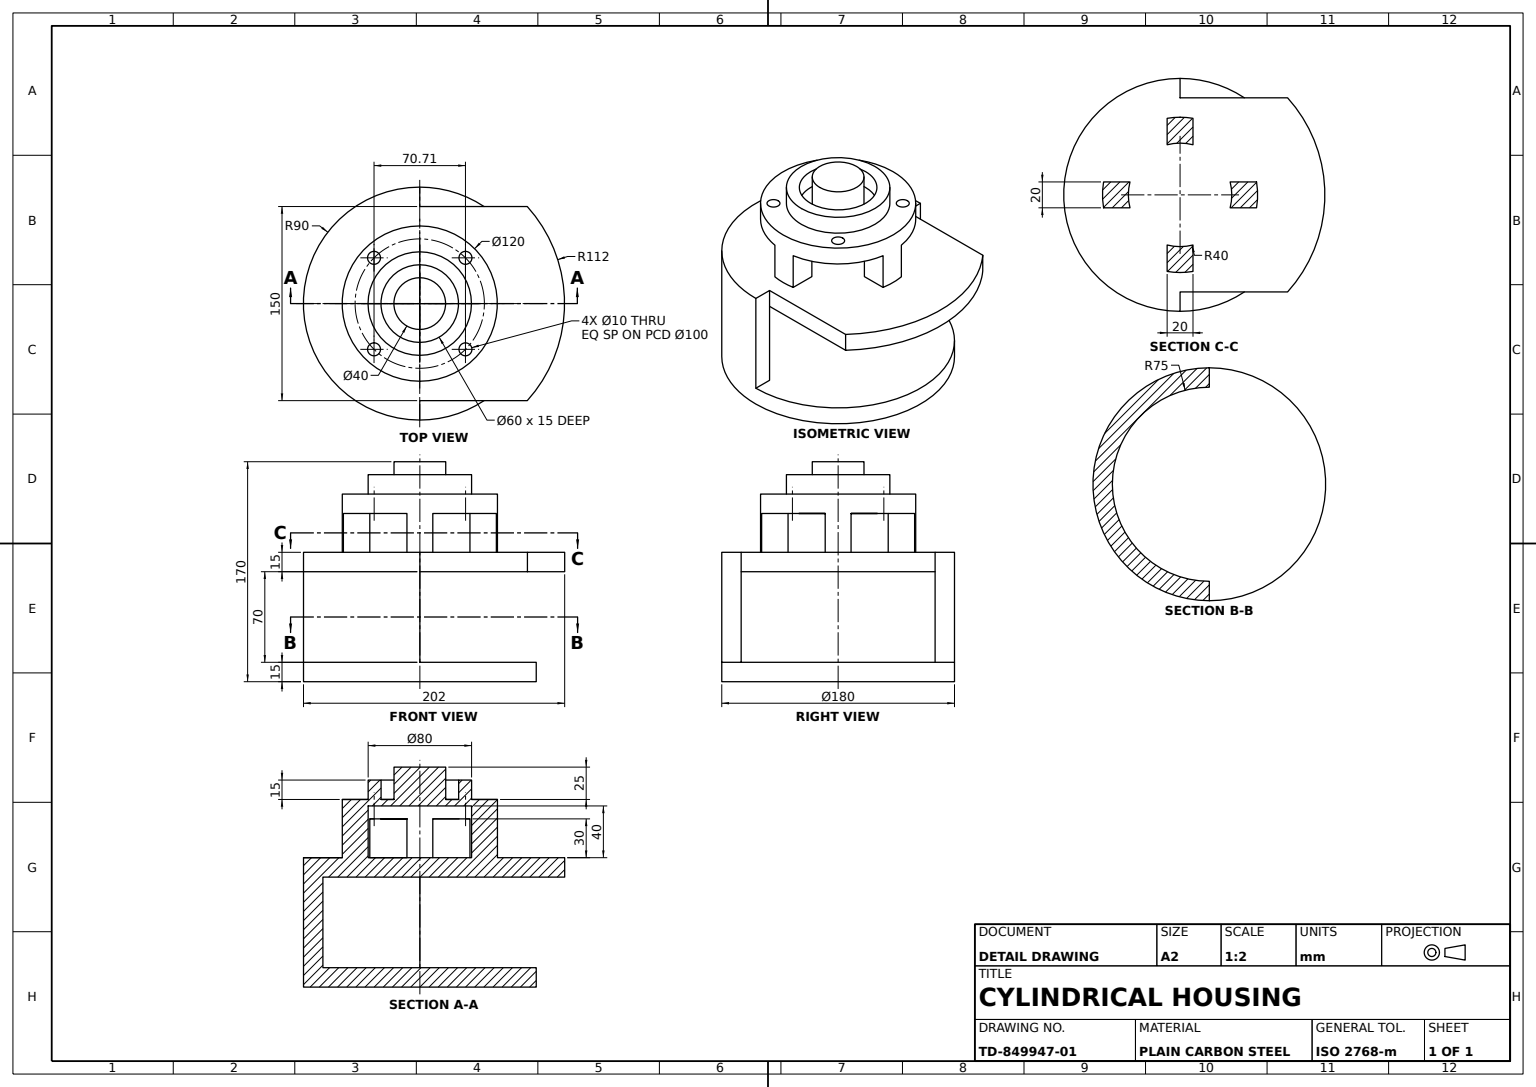
SolidWorks part; units mm, degrees
material "Plain Carbon Steel"
ref_plane "Front Plane" through (0, 0, 0) normal (0, 0, 1) x (1, 0, 0)
ref_plane "Top Plane" through (0, 0, 0) normal (0, 1, 0) x (1, 0, 0)
ref_plane "Right Plane" through (0, 0, 0) normal (1, 0, 0) x (0, 0, -1)
sketch "Base Disc Sketch" plane through (0, 0, 0) normal (0, 1, 0) x (1, 0, 0)
  circle A0 centre (0, 0) radius 90
  dimension "D1" = 180
extrude "Base Disc Ø180" add sketch "Base Disc Sketch" along normal blind 15
sketch "Clamp Frame Wall Sketch" plane through (0, 15, 0) normal (0, 1, 0) x (1, 0, 0)
  line L0 (0, -90) -> (0, -75)
  line L1 (0, 75) -> (0, 90)
  arc A0 (0, 90) -> (0, -90) centre (0, 0) ccw
  arc A1 (0, 75) -> (0, -75) centre (0, 0) ccw
  dimension "D1" = 150
  dimension "D2" = 180
extrude "Clamp Frame Wall" add sketch "Clamp Frame Wall Sketch" along normal blind 70
sketch "Top Jaw Sketch" plane through (0, 85, 0) normal (0, 1, 0) x (1, 0, 0)
  line L1 (0, 75) -> (83.1805, 75)
  line L2 (0, -75) -> (83.1805, -75)
  line L3 (0, -90) -> (0, 90)
  arc A0 (0, 90) -> (49.7494, -75) centre (0, 0) ccw
  arc A1 (0, 75) -> (0, -75) centre (0, 0) ccw
  arc A2 (83.1805, -75) -> (83.1805, 75) centre (0, 0) ccw
  point P9 (0, 0)
  arc M3 (0, 90) -> (0, -90) centre (0, 0) ccw
  line M4 (0, -90) -> (0, -75)
  arc M5 (0, -75) -> (0, 75) centre (0, 0) cw
  line M6 (0, 75) -> (0, 90)
  dimension "D1" = 180
  dimension "D2" = 83.1805
  dimension "D3" = 224
  dimension "D4" = 83.1805
extrude "Top Jaw Plate" add sketch "Top Jaw Sketch" along normal blind 15 contours M6 M3 M4 M5 | L3 M5 | L2 A2 L1 L3
sketch "Table Riser Sketch" plane through (0, 100, 0) normal (0, 1, 0) x (1, 0, 0)
  circle A0 centre (0, 0) radius 60
  circle A1 centre (0, 0) radius 40
  dimension "D1" = 120
  dimension "D2" = 80
extrude "Table Riser" add sketch "Table Riser Sketch" along normal blind 40
ref_plane "Riser Slot Plane" through (0, 130, 0) normal (0, 1, 0) x (1, 0, 0)
sketch "Riser Slots Sketch" plane through (0, 130, 0) normal (0, 1, 0) x (1, 0, 0)
  line L0 (59.1608, 10) -> (38.7298, 10)
  line L1 (-10, 59.1608) -> (-10, 38.7298)
  line L2 (10, 59.1608) -> (10, 38.7298)
  line L3 (59.1608, -10) -> (38.7298, -10)
  line L4 (10, -59.1608) -> (10, -38.7298)
  line L5 (-10, -59.1608) -> (-10, -38.7298)
  line L6 (-59.1608, -10) -> (-38.7298, -10)
  line L7 (-59.1608, 10) -> (-38.7298, 10)
  arc A0 (-10, 38.7298) -> (-38.7298, 10) centre (0, 0) ccw
  arc A1 (-10, 59.1608) -> (-59.1608, 10) centre (0, 0) ccw
  arc A2 (10, -38.7298) -> (38.7298, -10) centre (0, 0) ccw
  arc A3 (10, -59.1608) -> (59.1608, -10) centre (0, 0) ccw
  arc A4 (-38.7298, -10) -> (-10, -38.7298) centre (0, 0) ccw
  arc A5 (-59.1608, -10) -> (-10, -59.1608) centre (0, 0) ccw
  arc A6 (38.7298, 10) -> (10, 38.7298) centre (0, 0) ccw
  arc A7 (59.1608, 10) -> (10, 59.1608) centre (0, 0) ccw
  point P4 (0, 68.2304)
  point P5 (-10, 68.2304)
  point P6 (-10, 0)
  point P7 (10, 68.2304)
  point P8 (10, 0)
  dimension "D1" = 120
  dimension "D2" = 80
  dimension "D3" = 20.431
  dimension "D4" = 20
  dimension "D5" = 59.1608
  dimension "D6" = 4
extrude "Riser Slots Cut" cut sketch "Riser Slots Sketch" against normal blind 30
sketch "Table Plate Sketch" plane through (0, 140, 0) normal (0, 1, 0) x (1, 0, 0)
  circle A1 centre (0, 0) radius 60
  dimension "D2" = 120
extrude "Table Plate Ø120" add sketch "Table Plate Sketch" along normal blind 5
sketch "Table Bolt Holes Sketch" plane through (0, 145, 0) normal (0, 1, 0) x (1, 0, 0)
  line L0 (0, 75) -> (0, 0)
  line L1 (0, 0) -> (140.7055, 0)
  line L2 (0, 0) -> (107.4576, 107.4576)
  circle A1 centre (35.3553, 35.3553) radius 5
  circle A2 centre (35.3553, -35.3553) radius 5
  circle A3 centre (-35.3553, -35.3553) radius 5
  circle A4 centre (-35.3553, 35.3553) radius 5
  circle A5 centre (0, 0) radius 60 construction
  dimension "D2" = 70.7107
  dimension "D3" = 10
  dimension "D1" = 45
  dimension "D5" = 35.3553
  dimension "D6" = 35.3553
  dimension "D7" = 35.3553
  dimension "D8" = 35.3553
  dimension "D9" = 107.4576
  dimension "D10" = 140.7055
  dimension "D11" = 75
  dimension "D12" = 107.4576
  dimension "D4" = 4
extrude "Table Bolt Holes 4xØ10" cut sketch "Table Bolt Holes Sketch" against normal blind 20 contours L2 A1 | L2 A1 | A4 | A3 | A2
sketch "Table Ring Sketch" plane through (0, 145, 0) normal (0, 1, 0) x (1, 0, 0)
  circle A0 centre (0, 0) radius 40
  circle A1 centre (0, 0) radius 30
  dimension "D1" = 80
  dimension "D2" = 60
extrude "Table Ring Ø80" add sketch "Table Ring Sketch" along normal blind 15
sketch "Centre Spigot Sketch" plane through (0, 145, 0) normal (0, 1, 0) x (1, 0, 0)
  circle A0 centre (0, 0) radius 20
  dimension "D1" = 40
extrude "Centre Spigot Ø40" add sketch "Centre Spigot Sketch" along normal blind 25
